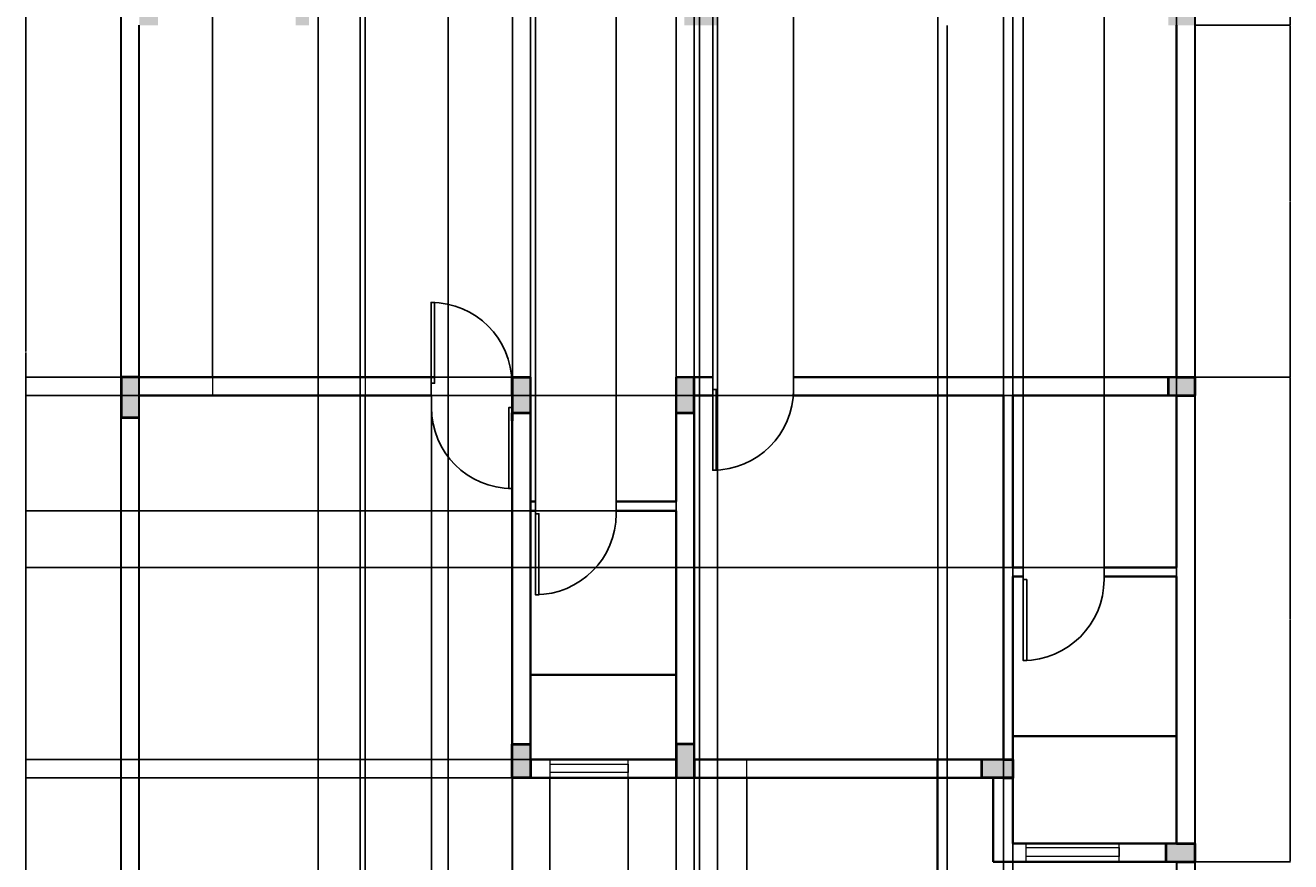
# Model space of a CAD drawing. Units: inches. Extents: x 1210 to 1836, y 84 to 1122.
# Tile 2 of 5: x 1210 to 1836, y 351 to 764. Entities that reach past the tile are written whole.
import ezdxf

# ---------------------------------------------------------------- set-up
doc = ezdxf.new("R2010")
doc.units = ezdxf.units.IN
doc.header["$MEASUREMENT"] = 0
for name, color, linetype, lineweight in [('A-ANNO-DIMS', 2, 'Continuous', 18), ('A-COLS', 7, 'Continuous', 40), ('A-COLS-PATT', 6, 'Continuous', 13), ('A-GLAZ', 4, 'Continuous', 18), ('A-WALL', 7, 'Continuous', 35), ('C-PROP', 32, 'Continuous', 30), ('DOORS', 24, 'Continuous', 25)]:
    doc.layers.add(name, color=color, linetype=linetype, lineweight=lineweight)
doc.styles.get("Standard").update_dxf_attribs({"font": 'arial.ttf'})
doc.dimstyles.get("Standard").update_dxf_attribs({"dimtxt": 0.18, "dimasz": 0.18, "dimexe": 0.18, "dimexo": 0.0625, "dimgap": 0.09, "dimtad": 0, "dimtih": 1, "dimtoh": 1, "dimdec": 4, "dimzin": 0, "dimdsep": 46, "dimtxsty": 'Standard', "dimcen": 0.09, "dimadec": 0, "dimazin": 0, "dimtfac": 1, "dimtdec": 4, "dimtofl": 0, "dimtmove": 0, "dimatfit": 3, "dimfxl": 1, "dimtolj": 1, "dimtzin": 0, "dimarcsym": 0})

# ---------------------------------------------------------------- blocks, each defined once
blk = doc.blocks.new('*U2')
for p, q in [((0, 0), (0, -6)), ((40, 0), (40, -6))]:
    blk.add_line(p, q)
blk.add_lwpolyline([(0, 0), (0, 40), (1.75, 40), (1.75, 0)], close=True)
blk.add_arc((0, 0), 40, 0, 90)
blk = doc.blocks.new('*U5')
for p, q in [((-40, 0), (-40, 6)), ((0, 0), (0, 6))]:
    blk.add_line(p, q)
blk.add_lwpolyline([(0, 0), (0, -40), (-1.75, -40), (-1.75, 0)], close=True)
blk.add_arc((0, 0), 40, 180, 270)
blk = doc.blocks.new('*U4')
for p, q in [((0, 0), (0, 6)), ((40, 0), (40, 6))]:
    blk.add_line(p, q)
blk.add_lwpolyline([(0, 0), (0, -40), (1.75, -40), (1.75, 0)], close=True)
blk.add_arc((0, 0), 40, 270, 0)
blk = doc.blocks.new('*D23')
at = {"layer": 'A-ANNO-DIMS', "color": 0, "lineweight": -2, "transparency": 16777216}
for p, q in [((1257.26, 1074.21), (1209.97, 1074.21)), ((1210.15, 1074.03), (1210.15, 602.9)), ((1210.15, 131.39), (1210.15, 602.53)), ((1257.26, 131.21), (1209.97, 131.21))]:
    blk.add_line(p, q, dxfattribs=at)
at = {"layer": 'A-ANNO-DIMS', "color": 0, "transparency": 16777216}
for points in [[(1210.12, 1074.03), (1210.18, 1074.03), (1210.15, 1074.21)], [(1210.12, 131.39), (1210.18, 131.39), (1210.15, 131.21)]]:
    blk.add_solid(points, dxfattribs=at)
at = {"layer": 'Defpoints', "color": 0, "transparency": 16777216}
for p in [(1210.15, 1074.21), (1257.32, 1074.21), (1257.32, 131.21)]:
    blk.add_point(p, dxfattribs=at)
at = {"layer": 'A-ANNO-DIMS', "color": 0, "transparency": 16777216, "insert": (1210.15, 602.71), "char_height": 0.18, "attachment_point": 5}
blk.add_mtext('\\A1;943', dxfattribs=at)
blk = doc.blocks.new('*D25')
at = {"layer": 'A-ANNO-DIMS', "color": 0, "lineweight": -2, "transparency": 16777216}
for p, q in [((1788.39, 938.21), (1835.68, 938.21)), ((1835.5, 938.03), (1835.5, 851.39)), ((1835.5, 764.39), (1835.5, 851.03)), ((1788.39, 764.21), (1835.68, 764.21))]:
    blk.add_line(p, q, dxfattribs=at)
at = {"layer": 'A-ANNO-DIMS', "color": 0, "transparency": 16777216}
for points in [[(1835.47, 938.03), (1835.53, 938.03), (1835.5, 938.21)], [(1835.47, 764.39), (1835.53, 764.39), (1835.5, 764.21)]]:
    blk.add_solid(points, dxfattribs=at)
at = {"layer": 'Defpoints', "color": 0, "transparency": 16777216}
for p in [(1788.32, 938.21), (1788.32, 764.21), (1835.5, 764.21)]:
    blk.add_point(p, dxfattribs=at)
at = {"layer": 'A-ANNO-DIMS', "color": 0, "transparency": 16777216, "insert": (1835.5, 851.21), "char_height": 0.18, "attachment_point": 5}
blk.add_mtext('\\A1;174', dxfattribs=at)
blk = doc.blocks.new('*D26')
at = {"layer": 'A-ANNO-DIMS', "color": 0, "lineweight": -2, "transparency": 16777216}
for p, q in [((1788.39, 764.21), (1835.68, 764.21)), ((1835.5, 764.03), (1835.5, 677.39)), ((1835.5, 590.39), (1835.5, 677.03)), ((1788.39, 590.21), (1835.68, 590.21))]:
    blk.add_line(p, q, dxfattribs=at)
at = {"layer": 'A-ANNO-DIMS', "color": 0, "transparency": 16777216}
for points in [[(1835.47, 764.03), (1835.53, 764.03), (1835.5, 764.21)], [(1835.47, 590.39), (1835.53, 590.39), (1835.5, 590.21)]]:
    blk.add_solid(points, dxfattribs=at)
at = {"layer": 'Defpoints', "color": 0, "transparency": 16777216}
for p in [(1788.32, 764.21), (1788.32, 590.21), (1835.5, 590.21)]:
    blk.add_point(p, dxfattribs=at)
at = {"layer": 'A-ANNO-DIMS', "color": 0, "transparency": 16777216, "insert": (1835.5, 677.21), "char_height": 0.18, "attachment_point": 5}
blk.add_mtext('\\A1;174', dxfattribs=at)
blk = doc.blocks.new('*D27')
at = {"layer": 'A-ANNO-DIMS', "color": 0, "lineweight": -2, "transparency": 16777216}
for p, q in [((1788.39, 590.21), (1835.68, 590.21)), ((1835.5, 590.03), (1835.5, 470.65)), ((1835.5, 350.89), (1835.5, 470.28)), ((1788.39, 350.71), (1835.68, 350.71))]:
    blk.add_line(p, q, dxfattribs=at)
at = {"layer": 'A-ANNO-DIMS', "color": 0, "transparency": 16777216}
for points in [[(1835.47, 590.03), (1835.53, 590.03), (1835.5, 590.21)], [(1835.47, 350.89), (1835.53, 350.89), (1835.5, 350.71)]]:
    blk.add_solid(points, dxfattribs=at)
at = {"layer": 'Defpoints', "color": 0, "transparency": 16777216}
for p in [(1788.32, 590.21), (1788.32, 350.71), (1835.5, 350.71)]:
    blk.add_point(p, dxfattribs=at)
at = {"layer": 'A-ANNO-DIMS', "color": 0, "transparency": 16777216, "insert": (1835.5, 470.46), "char_height": 0.18, "attachment_point": 5}
blk.add_mtext('\\A1;239.5', dxfattribs=at)
blk = doc.blocks.new('*D36')
at = {"layer": 'A-ANNO-DIMS', "color": 0, "lineweight": -2, "transparency": 16777216}
for p, q in [((1552.32, 840.82), (1552.32, 83.86)), ((1661.32, 840.82), (1661.32, 83.86)), ((1552.5, 84.04), (1606.54, 84.04)), ((1661.14, 84.04), (1607.1, 84.04))]:
    blk.add_line(p, q, dxfattribs=at)
at = {"layer": 'A-ANNO-DIMS', "color": 0, "transparency": 16777216}
for points in [[(1552.5, 84.07), (1552.5, 84.01), (1552.32, 84.04)], [(1661.14, 84.07), (1661.14, 84.01), (1661.32, 84.04)]]:
    blk.add_solid(points, dxfattribs=at)
at = {"layer": 'Defpoints', "color": 0, "transparency": 16777216}
for p in [(1552.32, 840.89), (1661.32, 840.89), (1661.32, 84.04)]:
    blk.add_point(p, dxfattribs=at)
at = {"layer": 'A-ANNO-DIMS', "color": 0, "transparency": 16777216, "insert": (1606.82, 84.04), "char_height": 0.18, "attachment_point": 5}
blk.add_mtext('\\A1;109', dxfattribs=at)
blk = doc.blocks.new('*D39')
at = {"layer": 'A-ANNO-DIMS', "color": 0, "lineweight": -2, "transparency": 16777216}
for p, q in [((1354.82, 773.15), (1354.82, 83.86)), ((1543.32, 773.15), (1543.32, 83.86)), ((1355, 84.04), (1448.69, 84.04)), ((1543.14, 84.04), (1449.46, 84.04))]:
    blk.add_line(p, q, dxfattribs=at)
at = {"layer": 'A-ANNO-DIMS', "color": 0, "transparency": 16777216}
for points in [[(1355, 84.07), (1355, 84.01), (1354.82, 84.04)], [(1543.14, 84.07), (1543.14, 84.01), (1543.32, 84.04)]]:
    blk.add_solid(points, dxfattribs=at)
at = {"layer": 'Defpoints', "color": 0, "transparency": 16777216}
for p in [(1354.82, 773.21), (1543.32, 773.21), (1543.32, 84.04)]:
    blk.add_point(p, dxfattribs=at)
at = {"layer": 'A-ANNO-DIMS', "color": 0, "transparency": 16777216, "insert": (1449.07, 84.04), "char_height": 0.18, "attachment_point": 5}
blk.add_mtext('\\A1;188.5', dxfattribs=at)
blk = doc.blocks.new('*D47')
at = {"layer": 'A-ANNO-DIMS', "color": 0, "lineweight": -2, "transparency": 16777216}
for p, q in [((1375.61, 773.15), (1375.61, 83.86)), ((1419.01, 773.15), (1419.01, 83.86)), ((1375.79, 84.04), (1396.98, 84.04)), ((1418.83, 84.04), (1397.64, 84.04))]:
    blk.add_line(p, q, dxfattribs=at)
at = {"layer": 'A-ANNO-DIMS', "color": 0, "transparency": 16777216}
for points in [[(1375.79, 84.07), (1375.79, 84.01), (1375.61, 84.04)], [(1418.83, 84.07), (1418.83, 84.01), (1419.01, 84.04)]]:
    blk.add_solid(points, dxfattribs=at)
at = {"layer": 'Defpoints', "color": 0, "transparency": 16777216}
for p in [(1375.61, 773.21), (1419.01, 773.21), (1419.01, 84.04)]:
    blk.add_point(p, dxfattribs=at)
at = {"layer": 'A-ANNO-DIMS', "color": 0, "transparency": 16777216, "insert": (1397.31, 84.04), "char_height": 0.18, "attachment_point": 5}
blk.add_mtext('\\A1;43.4', dxfattribs=at)
blk = doc.blocks.new('*D48')
at = {"layer": 'A-ANNO-DIMS', "color": 0, "lineweight": -2, "transparency": 16777216}
for p, q in [((1419.01, 773.15), (1419.01, 83.86)), ((1450.89, 772.94), (1450.89, 83.86)), ((1419.19, 84.04), (1434.55, 84.04)), ((1450.71, 84.04), (1435.34, 84.04))]:
    blk.add_line(p, q, dxfattribs=at)
at = {"layer": 'A-ANNO-DIMS', "color": 0, "transparency": 16777216}
for points in [[(1419.19, 84.07), (1419.19, 84.01), (1419.01, 84.04)], [(1450.71, 84.07), (1450.71, 84.01), (1450.89, 84.04)]]:
    blk.add_solid(points, dxfattribs=at)
at = {"layer": 'Defpoints', "color": 0, "transparency": 16777216}
for p in [(1419.01, 773.21), (1450.89, 773), (1450.89, 84.04)]:
    blk.add_point(p, dxfattribs=at)
at = {"layer": 'A-ANNO-DIMS', "color": 0, "transparency": 16777216, "insert": (1434.95, 84.04), "char_height": 0.18, "attachment_point": 5}
blk.add_mtext('\\A1;31.88', dxfattribs=at)
blk = doc.blocks.new('*D57')
at = {"layer": 'A-ANNO-DIMS', "color": 0, "lineweight": -2, "transparency": 16777216}
for p, q in [((1552.32, 764.15), (1552.32, 83.86)), ((1665.82, 764.15), (1665.82, 83.86)), ((1552.5, 84.04), (1608.69, 84.04)), ((1665.64, 84.04), (1609.46, 84.04))]:
    blk.add_line(p, q, dxfattribs=at)
at = {"layer": 'A-ANNO-DIMS', "color": 0, "transparency": 16777216}
for points in [[(1552.5, 84.07), (1552.5, 84.01), (1552.32, 84.04)], [(1665.64, 84.07), (1665.64, 84.01), (1665.82, 84.04)]]:
    blk.add_solid(points, dxfattribs=at)
at = {"layer": 'Defpoints', "color": 0, "transparency": 16777216}
for p in [(1552.32, 764.21), (1665.82, 764.21), (1665.82, 84.04)]:
    blk.add_point(p, dxfattribs=at)
at = {"layer": 'A-ANNO-DIMS', "color": 0, "transparency": 16777216, "insert": (1609.07, 84.04), "char_height": 0.18, "attachment_point": 5}
blk.add_mtext('\\A1;113.5', dxfattribs=at)
blk = doc.blocks.new('*D59')
at = {"layer": 'A-ANNO-DIMS', "color": 0, "lineweight": -2, "transparency": 16777216}
for p, q in [((1459.82, 443.21), (1459.82, 1121.57)), ((1460, 1121.39), (1495.61, 1121.39)), ((1531.64, 1121.39), (1496.04, 1121.39)), ((1531.82, 443.21), (1531.82, 1121.57))]:
    blk.add_line(p, q, dxfattribs=at)
at = {"layer": 'A-ANNO-DIMS', "color": 0, "transparency": 16777216}
for points in [[(1460, 1121.42), (1460, 1121.36), (1459.82, 1121.39)], [(1531.64, 1121.42), (1531.64, 1121.36), (1531.82, 1121.39)]]:
    blk.add_solid(points, dxfattribs=at)
at = {"layer": 'Defpoints', "color": 0, "transparency": 16777216}
for p in [(1531.82, 1121.39), (1459.82, 443.15), (1531.82, 443.15)]:
    blk.add_point(p, dxfattribs=at)
at = {"layer": 'A-ANNO-DIMS', "color": 0, "transparency": 16777216, "insert": (1495.82, 1121.39), "char_height": 0.18, "attachment_point": 5}
blk.add_mtext('\\A1;72', dxfattribs=at)
blk = doc.blocks.new('*D60')
at = {"layer": 'A-ANNO-DIMS', "color": 0, "lineweight": -2, "transparency": 16777216}
for p, q in [((1540.82, 401.28), (1540.82, 1121.57)), ((1541, 1121.39), (1617.04, 1121.39)), ((1693.64, 1121.39), (1617.6, 1121.39)), ((1693.82, 401.28), (1693.82, 1121.57))]:
    blk.add_line(p, q, dxfattribs=at)
at = {"layer": 'A-ANNO-DIMS', "color": 0, "transparency": 16777216}
for points in [[(1541, 1121.42), (1541, 1121.36), (1540.82, 1121.39)], [(1693.64, 1121.42), (1693.64, 1121.36), (1693.82, 1121.39)]]:
    blk.add_solid(points, dxfattribs=at)
at = {"layer": 'Defpoints', "color": 0, "transparency": 16777216}
for p in [(1693.82, 1121.39), (1540.82, 401.21), (1693.82, 401.21)]:
    blk.add_point(p, dxfattribs=at)
at = {"layer": 'A-ANNO-DIMS', "color": 0, "transparency": 16777216, "insert": (1617.32, 1121.39), "char_height": 0.18, "attachment_point": 5}
blk.add_mtext('\\A1;153', dxfattribs=at)
blk = doc.blocks.new('*D61')
at = {"layer": 'A-ANNO-DIMS', "color": 0, "lineweight": -2, "transparency": 16777216}
for p, q in [((1698.32, 412.85), (1698.32, 1121.57)), ((1698.5, 1121.39), (1738.62, 1121.39)), ((1779.14, 1121.39), (1739.03, 1121.39)), ((1779.32, 412.85), (1779.32, 1121.57))]:
    blk.add_line(p, q, dxfattribs=at)
at = {"layer": 'A-ANNO-DIMS', "color": 0, "transparency": 16777216}
for points in [[(1698.5, 1121.42), (1698.5, 1121.36), (1698.32, 1121.39)], [(1779.14, 1121.42), (1779.14, 1121.36), (1779.32, 1121.39)]]:
    blk.add_solid(points, dxfattribs=at)
at = {"layer": 'Defpoints', "color": 0, "transparency": 16777216}
for p in [(1779.32, 1121.39), (1698.32, 412.79), (1779.32, 412.79)]:
    blk.add_point(p, dxfattribs=at)
at = {"layer": 'A-ANNO-DIMS', "color": 0, "transparency": 16777216, "insert": (1738.82, 1121.39), "char_height": 0.18, "attachment_point": 5}
blk.add_mtext('\\A1;81', dxfattribs=at)
blk = doc.blocks.new('*D62')
at = {"layer": 'A-ANNO-DIMS', "color": 0, "lineweight": -2, "transparency": 16777216}
for p, q in [((1450.76, 590.21), (1209.97, 590.21)), ((1210.15, 590.03), (1210.15, 491.4)), ((1210.15, 392.39), (1210.15, 491.03)), ((1450.76, 392.21), (1209.97, 392.21))]:
    blk.add_line(p, q, dxfattribs=at)
at = {"layer": 'A-ANNO-DIMS', "color": 0, "transparency": 16777216}
for points in [[(1210.12, 590.03), (1210.18, 590.03), (1210.15, 590.21)], [(1210.12, 392.39), (1210.18, 392.39), (1210.15, 392.21)]]:
    blk.add_solid(points, dxfattribs=at)
at = {"layer": 'Defpoints', "color": 0, "transparency": 16777216}
for p in [(1210.15, 590.21), (1450.82, 590.21), (1450.82, 392.21)]:
    blk.add_point(p, dxfattribs=at)
at = {"layer": 'A-ANNO-DIMS', "color": 0, "transparency": 16777216, "insert": (1210.15, 491.21), "char_height": 0.18, "attachment_point": 5}
blk.add_mtext('\\A1;198', dxfattribs=at)
blk = doc.blocks.new('*D63')
at = {"layer": 'A-ANNO-DIMS', "color": 0, "lineweight": -2, "transparency": 16777216}
for p, q in [((1531.76, 524.21), (1209.97, 524.21)), ((1210.15, 524.03), (1210.15, 462.9)), ((1210.15, 401.39), (1210.15, 462.53)), ((1531.76, 401.21), (1209.97, 401.21))]:
    blk.add_line(p, q, dxfattribs=at)
at = {"layer": 'A-ANNO-DIMS', "color": 0, "transparency": 16777216}
for points in [[(1210.12, 524.03), (1210.18, 524.03), (1210.15, 524.21)], [(1210.12, 401.39), (1210.18, 401.39), (1210.15, 401.21)]]:
    blk.add_solid(points, dxfattribs=at)
at = {"layer": 'Defpoints', "color": 0, "transparency": 16777216}
for p in [(1210.15, 524.21), (1531.82, 524.21), (1531.82, 401.21)]:
    blk.add_point(p, dxfattribs=at)
at = {"layer": 'A-ANNO-DIMS', "color": 0, "transparency": 16777216, "insert": (1210.15, 462.71), "char_height": 0.18, "attachment_point": 5}
blk.add_mtext('\\A1;123', dxfattribs=at)
blk = doc.blocks.new('*D64')
at = {"layer": 'A-ANNO-DIMS', "color": 0, "lineweight": -2, "transparency": 16777216}
for p, q in [((1779.26, 581.21), (1209.97, 581.21)), ((1210.15, 581.03), (1210.15, 538.9)), ((1210.15, 496.39), (1210.15, 538.53)), ((1779.26, 496.21), (1209.97, 496.21))]:
    blk.add_line(p, q, dxfattribs=at)
at = {"layer": 'A-ANNO-DIMS', "color": 0, "transparency": 16777216}
for points in [[(1210.12, 581.03), (1210.18, 581.03), (1210.15, 581.21)], [(1210.12, 496.39), (1210.18, 496.39), (1210.15, 496.21)]]:
    blk.add_solid(points, dxfattribs=at)
at = {"layer": 'Defpoints', "color": 0, "transparency": 16777216}
for p in [(1210.15, 581.21), (1779.32, 581.21), (1779.32, 496.21)]:
    blk.add_point(p, dxfattribs=at)
at = {"layer": 'A-ANNO-DIMS', "color": 0, "transparency": 16777216, "insert": (1210.15, 538.71), "char_height": 0.18, "attachment_point": 5}
blk.add_mtext('\\A1;85', dxfattribs=at)
blk = doc.blocks.new('*D65')
at = {"layer": 'A-ANNO-DIMS', "color": 0, "lineweight": -2, "transparency": 16777216}
for p, q in [((1549.93, 581.28), (1549.93, 1121.57)), ((1550.11, 1121.39), (1569.48, 1121.39)), ((1589.64, 1121.39), (1570.27, 1121.39)), ((1589.82, 581.28), (1589.82, 1121.57))]:
    blk.add_line(p, q, dxfattribs=at)
at = {"layer": 'A-ANNO-DIMS', "color": 0, "transparency": 16777216}
for points in [[(1550.11, 1121.42), (1550.11, 1121.36), (1549.93, 1121.39)], [(1589.64, 1121.42), (1589.64, 1121.36), (1589.82, 1121.39)]]:
    blk.add_solid(points, dxfattribs=at)
at = {"layer": 'Defpoints', "color": 0, "transparency": 16777216}
for p in [(1589.82, 1121.39), (1549.93, 581.21), (1589.82, 581.21)]:
    blk.add_point(p, dxfattribs=at)
at = {"layer": 'A-ANNO-DIMS', "color": 0, "transparency": 16777216, "insert": (1569.88, 1121.39), "char_height": 0.18, "attachment_point": 5}
blk.add_mtext('\\A1;39.89', dxfattribs=at)
blk = doc.blocks.new('*D66')
at = {"layer": 'A-ANNO-DIMS', "color": 0, "lineweight": -2, "transparency": 16777216}
for p, q in [((1508.09, 392.15), (1508.09, 83.86)), ((1531.82, 392.15), (1531.82, 83.86)), ((1508.27, 84.04), (1519.56, 84.04)), ((1531.64, 84.04), (1520.35, 84.04))]:
    blk.add_line(p, q, dxfattribs=at)
at = {"layer": 'A-ANNO-DIMS', "color": 0, "transparency": 16777216}
for points in [[(1508.27, 84.07), (1508.27, 84.01), (1508.09, 84.04)], [(1531.64, 84.07), (1531.64, 84.01), (1531.82, 84.04)]]:
    blk.add_solid(points, dxfattribs=at)
at = {"layer": 'Defpoints', "color": 0, "transparency": 16777216}
for p in [(1508.09, 392.21), (1531.82, 392.21), (1531.82, 84.04)]:
    blk.add_point(p, dxfattribs=at)
at = {"layer": 'A-ANNO-DIMS', "color": 0, "transparency": 16777216, "insert": (1519.96, 84.04), "char_height": 0.18, "attachment_point": 5}
blk.add_mtext('\\A1;23.73', dxfattribs=at)
blk = doc.blocks.new('*D67')
at = {"layer": 'A-ANNO-DIMS', "color": 0, "lineweight": -2, "transparency": 16777216}
for p, q in [((1469.4, 392.15), (1469.4, 83.86)), ((1508.09, 392.15), (1508.09, 83.86)), ((1469.58, 84.04), (1488.42, 84.04)), ((1507.91, 84.04), (1489.07, 84.04))]:
    blk.add_line(p, q, dxfattribs=at)
at = {"layer": 'A-ANNO-DIMS', "color": 0, "transparency": 16777216}
for points in [[(1469.58, 84.07), (1469.58, 84.01), (1469.4, 84.04)], [(1507.91, 84.07), (1507.91, 84.01), (1508.09, 84.04)]]:
    blk.add_solid(points, dxfattribs=at)
at = {"layer": 'Defpoints', "color": 0, "transparency": 16777216}
for p in [(1469.4, 392.21), (1508.09, 392.21), (1508.09, 84.04)]:
    blk.add_point(p, dxfattribs=at)
at = {"layer": 'A-ANNO-DIMS', "color": 0, "transparency": 16777216, "insert": (1488.75, 84.04), "char_height": 0.18, "attachment_point": 5}
blk.add_mtext('\\A1;38.7', dxfattribs=at)
blk = doc.blocks.new('*D68')
at = {"layer": 'A-ANNO-DIMS', "color": 0, "lineweight": -2, "transparency": 16777216}
for p, q in [((1540.82, 392.15), (1540.82, 83.86)), ((1566.82, 392.15), (1566.82, 83.86)), ((1541, 84.04), (1553.42, 84.04)), ((1566.64, 84.04), (1554.22, 84.04))]:
    blk.add_line(p, q, dxfattribs=at)
at = {"layer": 'A-ANNO-DIMS', "color": 0, "transparency": 16777216}
for points in [[(1541, 84.07), (1541, 84.01), (1540.82, 84.04)], [(1566.64, 84.07), (1566.64, 84.01), (1566.82, 84.04)]]:
    blk.add_solid(points, dxfattribs=at)
at = {"layer": 'Defpoints', "color": 0, "transparency": 16777216}
for p in [(1540.82, 392.21), (1566.82, 392.21), (1566.82, 84.04)]:
    blk.add_point(p, dxfattribs=at)
at = {"layer": 'A-ANNO-DIMS', "color": 0, "transparency": 16777216, "insert": (1553.82, 84.04), "char_height": 0.18, "attachment_point": 5}
blk.add_mtext('\\A1;25.99', dxfattribs=at)
blk = doc.blocks.new('*D69')
at = {"layer": 'A-ANNO-DIMS', "color": 0, "lineweight": -2, "transparency": 16777216}
for p, q in [((1566.82, 392.15), (1566.82, 83.86)), ((1660.99, 392.15), (1660.99, 83.86)), ((1567, 84.04), (1613.51, 84.04)), ((1660.81, 84.04), (1614.29, 84.04))]:
    blk.add_line(p, q, dxfattribs=at)
at = {"layer": 'A-ANNO-DIMS', "color": 0, "transparency": 16777216}
for points in [[(1567, 84.07), (1567, 84.01), (1566.82, 84.04)], [(1660.81, 84.07), (1660.81, 84.01), (1660.99, 84.04)]]:
    blk.add_solid(points, dxfattribs=at)
at = {"layer": 'Defpoints', "color": 0, "transparency": 16777216}
for p in [(1566.82, 392.21), (1660.99, 392.21), (1660.99, 84.04)]:
    blk.add_point(p, dxfattribs=at)
at = {"layer": 'A-ANNO-DIMS', "color": 0, "transparency": 16777216, "insert": (1613.9, 84.04), "char_height": 0.18, "attachment_point": 5}
blk.add_mtext('\\A1;94.17', dxfattribs=at)
blk = doc.blocks.new('*D72')
at = {"layer": 'A-ANNO-DIMS', "color": 0, "lineweight": -2, "transparency": 16777216}
for p, q in [((1257.32, 590.28), (1257.32, 1121.57)), ((1257.5, 1121.39), (1279.44, 1121.39)), ((1302.31, 1121.39), (1280.37, 1121.39)), ((1302.49, 590.28), (1302.49, 1121.57))]:
    blk.add_line(p, q, dxfattribs=at)
at = {"layer": 'A-ANNO-DIMS', "color": 0, "transparency": 16777216}
for points in [[(1257.5, 1121.42), (1257.5, 1121.36), (1257.32, 1121.39)], [(1302.31, 1121.42), (1302.31, 1121.36), (1302.49, 1121.39)]]:
    blk.add_solid(points, dxfattribs=at)
at = {"layer": 'Defpoints', "color": 0, "transparency": 16777216}
for p in [(1302.49, 1121.39), (1257.32, 590.21), (1302.49, 590.21)]:
    blk.add_point(p, dxfattribs=at)
at = {"layer": 'A-ANNO-DIMS', "color": 0, "transparency": 16777216, "insert": (1279.91, 1121.39), "char_height": 0.18, "attachment_point": 5}
blk.add_mtext('\\A1;45.165', dxfattribs=at)
blk = doc.blocks.new('*D73')
at = {"layer": 'A-ANNO-DIMS', "color": 0, "lineweight": -2, "transparency": 16777216}
for p, q in [((1302.49, 590.28), (1302.49, 1121.57)), ((1302.67, 1121.39), (1339.91, 1121.39)), ((1377.81, 1121.39), (1340.56, 1121.39)), ((1377.99, 590.28), (1377.99, 1121.57))]:
    blk.add_line(p, q, dxfattribs=at)
at = {"layer": 'A-ANNO-DIMS', "color": 0, "transparency": 16777216}
for points in [[(1302.67, 1121.42), (1302.67, 1121.36), (1302.49, 1121.39)], [(1377.81, 1121.42), (1377.81, 1121.36), (1377.99, 1121.39)]]:
    blk.add_solid(points, dxfattribs=at)
at = {"layer": 'Defpoints', "color": 0, "transparency": 16777216}
for p in [(1377.99, 1121.39), (1302.49, 590.21), (1377.99, 590.21)]:
    blk.add_point(p, dxfattribs=at)
at = {"layer": 'A-ANNO-DIMS', "color": 0, "transparency": 16777216, "insert": (1340.24, 1121.39), "char_height": 0.18, "attachment_point": 5}
blk.add_mtext('\\A1;75.5', dxfattribs=at)
blk = doc.blocks.new('*D74')
at = {"layer": 'A-ANNO-DIMS', "color": 0, "lineweight": -2, "transparency": 16777216}
for p, q in [((1377.99, 581.15), (1377.99, 83.86)), ((1410.82, 581.15), (1410.82, 83.86)), ((1378.17, 84.04), (1394.01, 84.04)), ((1410.64, 84.04), (1394.8, 84.04))]:
    blk.add_line(p, q, dxfattribs=at)
at = {"layer": 'A-ANNO-DIMS', "color": 0, "transparency": 16777216}
for points in [[(1378.17, 84.07), (1378.17, 84.01), (1377.99, 84.04)], [(1410.64, 84.07), (1410.64, 84.01), (1410.82, 84.04)]]:
    blk.add_solid(points, dxfattribs=at)
at = {"layer": 'Defpoints', "color": 0, "transparency": 16777216}
for p in [(1377.99, 581.21), (1410.82, 581.21), (1410.82, 84.04)]:
    blk.add_point(p, dxfattribs=at)
at = {"layer": 'A-ANNO-DIMS', "color": 0, "transparency": 16777216, "insert": (1394.4, 84.04), "char_height": 0.18, "attachment_point": 5}
blk.add_mtext('\\A1;32.84', dxfattribs=at)
blk = doc.blocks.new('*D75')
at = {"layer": 'A-ANNO-DIMS', "color": 0, "lineweight": -2, "transparency": 16777216}
for p, q in [((1410.82, 575.15), (1410.82, 83.86)), ((1450.82, 575.15), (1450.82, 83.86)), ((1411, 84.04), (1430.6, 84.04)), ((1450.64, 84.04), (1431.05, 84.04))]:
    blk.add_line(p, q, dxfattribs=at)
at = {"layer": 'A-ANNO-DIMS', "color": 0, "transparency": 16777216}
for points in [[(1411, 84.07), (1411, 84.01), (1410.82, 84.04)], [(1450.64, 84.07), (1450.64, 84.01), (1450.82, 84.04)]]:
    blk.add_solid(points, dxfattribs=at)
at = {"layer": 'Defpoints', "color": 0, "transparency": 16777216}
for p in [(1410.82, 575.21), (1450.82, 575.21), (1450.82, 84.04)]:
    blk.add_point(p, dxfattribs=at)
at = {"layer": 'A-ANNO-DIMS', "color": 0, "transparency": 16777216, "insert": (1430.82, 84.04), "char_height": 0.18, "attachment_point": 5}
blk.add_mtext('\\A1;40', dxfattribs=at)
blk = doc.blocks.new('*D76')
at = {"layer": 'A-ANNO-DIMS', "color": 0, "lineweight": -2, "transparency": 16777216}
for p, q in [((1462.25, 528.78), (1462.25, 1121.57)), ((1462.43, 1121.39), (1482.03, 1121.39)), ((1502.07, 1121.39), (1482.47, 1121.39)), ((1502.25, 528.78), (1502.25, 1121.57))]:
    blk.add_line(p, q, dxfattribs=at)
at = {"layer": 'A-ANNO-DIMS', "color": 0, "transparency": 16777216}
for points in [[(1462.43, 1121.42), (1462.43, 1121.36), (1462.25, 1121.39)], [(1502.07, 1121.42), (1502.07, 1121.36), (1502.25, 1121.39)]]:
    blk.add_solid(points, dxfattribs=at)
at = {"layer": 'Defpoints', "color": 0, "transparency": 16777216}
for p in [(1502.25, 1121.39), (1462.25, 528.71), (1502.25, 528.71)]:
    blk.add_point(p, dxfattribs=at)
at = {"layer": 'A-ANNO-DIMS', "color": 0, "transparency": 16777216, "insert": (1482.25, 1121.39), "char_height": 0.18, "attachment_point": 5}
blk.add_mtext('\\A1;40', dxfattribs=at)
blk = doc.blocks.new('*D77')
at = {"layer": 'A-ANNO-DIMS', "color": 0, "lineweight": -2, "transparency": 16777216}
for p, q in [((1703.49, 496.28), (1703.49, 1121.57)), ((1703.67, 1121.39), (1723.26, 1121.39)), ((1743.31, 1121.39), (1723.71, 1121.39)), ((1743.49, 496.28), (1743.49, 1121.57))]:
    blk.add_line(p, q, dxfattribs=at)
at = {"layer": 'A-ANNO-DIMS', "color": 0, "transparency": 16777216}
for points in [[(1703.67, 1121.42), (1703.67, 1121.36), (1703.49, 1121.39)], [(1743.31, 1121.42), (1743.31, 1121.36), (1743.49, 1121.39)]]:
    blk.add_solid(points, dxfattribs=at)
at = {"layer": 'Defpoints', "color": 0, "transparency": 16777216}
for p in [(1743.49, 1121.39), (1703.49, 496.21), (1743.49, 496.21)]:
    blk.add_point(p, dxfattribs=at)
at = {"layer": 'A-ANNO-DIMS', "color": 0, "transparency": 16777216, "insert": (1723.49, 1121.39), "char_height": 0.18, "attachment_point": 5}
blk.add_mtext('\\A1;40', dxfattribs=at)
blk = doc.blocks.new('*D78')
at = {"layer": 'A-ANNO-DIMS', "color": 0, "lineweight": -2, "transparency": 16777216}
for p, q in [((1693.82, 581.15), (1693.82, 83.86)), ((1698.32, 581.15), (1698.32, 83.86)), ((1694, 84.04), (1695.82, 84.04)), ((1698.14, 84.04), (1696.33, 84.04))]:
    blk.add_line(p, q, dxfattribs=at)
at = {"layer": 'A-ANNO-DIMS', "color": 0, "transparency": 16777216}
for points in [[(1694, 84.07), (1694, 84.01), (1693.82, 84.04)], [(1698.14, 84.07), (1698.14, 84.01), (1698.32, 84.04)]]:
    blk.add_solid(points, dxfattribs=at)
at = {"layer": 'Defpoints', "color": 0, "transparency": 16777216}
for p in [(1693.82, 581.21), (1698.32, 581.21), (1698.32, 84.04)]:
    blk.add_point(p, dxfattribs=at)
at = {"layer": 'A-ANNO-DIMS', "color": 0, "transparency": 16777216, "insert": (1696.07, 84.04), "char_height": 0.18, "attachment_point": 5}
blk.add_mtext('\\A1;4.5', dxfattribs=at)

msp = doc.modelspace()

# ---------------------------------------------------------------- hatches: boundary and pattern name
at = {"layer": 'A-COLS-PATT'}
h = msp.add_hatch(color=256, dxfattribs=at)
h.dxf.hatch_style = 1
h.paths.add_polyline_path([(1266.3239, 938.214), (1257.3239, 938.214), (1257.3239, 929.4573), (1257.3239, 923.2025), (1266.3239, 923.2025)])
h.paths.add_polyline_path([(1350.3239, 929.214), (1350.3239, 938.214), (1339.1886, 938.214), (1339.1886, 929.214)])
h.paths.add_polyline_path([(1559.1961, 929.214), (1559.1961, 938.214), (1542.8626, 938.214), (1542.8626, 929.214), (1543.3239, 929.214)])
h.paths.add_polyline_path([(1771.5139, 938.214), (1771.5139, 929.214), (1788.3239, 929.214), (1788.3239, 938.214)])
h.paths.add_polyline_path([(1788.3239, 764.214), (1788.3239, 773.214), (1775.2119, 773.214), (1775.2119, 764.214)])
h.paths.add_polyline_path([(1552.3239, 764.214), (1552.3239, 773.214), (1543.3239, 773.214), (1535.8494, 773.197), (1535.8494, 764.214)])
h.paths.add_polyline_path([(1275.5217, 782.2138), (1272.7843, 782.2138), (1266.3239, 782.2138), (1266.3239, 764.214), (1275.5217, 764.214)])
h.paths.add_polyline_path([(1350.2372, 764.214), (1350.3239, 773.214), (1343.6352, 773.214), (1343.6352, 764.214)])
h.paths.add_polyline_path([(1257.3239, 570.3846), (1266.3239, 570.3846), (1266.3239, 590.214), (1257.3239, 590.214)])
h.paths.add_polyline_path([(1450.8239, 572.5809), (1459.8239, 572.5809), (1459.8239, 590.214), (1458.3239, 590.214), (1450.8239, 590.214)])
h.paths.add_polyline_path([(1531.8239, 572.5809), (1540.8239, 572.5809), (1540.8239, 590.214), (1531.8239, 590.214)])
h.paths.add_polyline_path([(1450.8239, 392.214), (1459.8239, 392.214), (1459.8239, 401.214), (1459.8239, 408.7866), (1450.8239, 408.7866)])
h.paths.add_polyline_path([(1531.8239, 392.214), (1540.8239, 392.214), (1540.8239, 401.214), (1540.8239, 408.7866), (1531.8239, 408.7866)])
h.paths.add_polyline_path([(1682.9725, 401.214), (1682.9725, 392.214), (1698.3239, 392.214), (1698.3239, 401.214), (1693.8239, 401.214)])
h.paths.add_polyline_path([(1774.197, 350.714), (1779.3239, 350.714), (1788.3239, 350.714), (1788.3239, 359.714), (1779.3239, 359.714), (1774.197, 359.714)])
h.paths.add_polyline_path([(1779.3239, 590.214), (1775.4485, 590.214), (1775.4485, 581.214), (1779.3239, 581.214), (1788.3239, 581.214), (1788.3239, 590.214)])

# ---------------------------------------------------------------- linework, layer by layer
at = {"layer": 'A-COLS'}
for p, q in [((1266.3239, 590.214), (1257.3239, 590.214)), ((1257.3239, 590.214), (1257.3239, 570.3846)), ((1450.4926, 590.214), (1458.3239, 590.214)), ((1450.8239, 581.214), (1450.8239, 590.214)), ((1450.8239, 590.214), (1450.8239, 568.7267)), ((1458.3239, 590.214), (1459.8239, 590.214)), ((1540.8239, 572.5809), (1540.8239, 590.214)), ((1775.4485, 581.214), (1775.4485, 590.214)), ((1779.3239, 590.214), (1788.3239, 590.214)), ((1788.3239, 590.214), (1788.3239, 581.1742)), ((1450.6052, 581.214), (1450.8239, 581.214)), ((1779.3239, 581.214), (1788.3239, 581.214)), ((1257.3239, 570.3846), (1266.3239, 570.3846)), ((1450.8239, 568.7267), (1450.8239, 572.5809)), ((1450.8239, 572.5809), (1459.8239, 572.5809)), ((1531.8239, 572.5809), (1540.8239, 572.5809)), ((1450.8239, 392.214), (1450.8239, 408.7866)), ((1450.8239, 408.7866), (1459.8239, 408.7866)), ((1540.8239, 408.7866), (1531.8239, 408.7866)), ((1531.8239, 408.7866), (1531.8239, 392.214)), ((1459.8239, 401.214), (1459.8239, 392.214)), ((1540.8239, 401.214), (1540.8239, 392.214)), ((1682.9725, 392.214), (1682.9725, 401.214)), ((1693.8239, 401.214), (1698.3239, 401.214)), ((1698.3239, 401.214), (1698.3239, 392.0825)), ((1459.8239, 392.214), (1450.8239, 392.214)), ((1698.3239, 392.214), (1682.9725, 392.214)), ((1693.8239, 392.214), (1698.3239, 392.214)), ((1774.197, 350.714), (1774.197, 359.714)), ((1779.3239, 359.714), (1788.3239, 359.714)), ((1788.3239, 359.714), (1788.3239, 350.8323)), ((1779.3239, 350.714), (1788.3239, 350.714))]:
    msp.add_line(p, q, dxfattribs=at)
at = {"layer": 'A-GLAZ'}
for p, q in [((1302.4894, 590.214), (1302.4894, 581.214)), ((1378.2066, 581.5192), (1378.2066, 590.5192)), ((1302.4894, 581.214), (1377.9853, 581.214)), ((1469.397, 401.214), (1469.397, 392.214)), ((1508.0938, 392.214), (1508.0938, 401.214)), ((1566.8155, 392.214), (1566.8155, 401.214)), ((1660.9867, 392.214), (1660.9867, 401.214)), ((1469.397, 398.974), (1508.0938, 398.974)), ((1508.0938, 394.8322), (1469.397, 394.8322)), ((1508.0938, 398.974), (1508.0938, 394.8322)), ((1704.8288, 359.714), (1704.8288, 350.714)), ((1704.8288, 359.714), (1704.8288, 357.757)), ((1704.8288, 357.757), (1750.8976, 357.757)), ((1750.8976, 350.714), (1750.8976, 359.714)), ((1750.8976, 357.757), (1750.8976, 355.214)), ((1750.8976, 353.3014), (1704.8288, 353.3014)), ((1704.8288, 350.714), (1750.8976, 350.714)), ((1750.8976, 355.214), (1750.8976, 353.3014))]:
    msp.add_line(p, q, dxfattribs=at)
at = {"layer": 'A-WALL'}
for p, q in [((1779.3239, 764.214), (1779.3239, 590.214)), ((1266.3239, 590.214), (1412.3552, 590.214)), ((1377.9853, 590.214), (1394.3053, 590.214)), ((1459.8239, 401.214), (1459.8239, 590.214)), ((1531.8239, 590.214), (1549.9335, 590.214)), ((1531.8239, 590.214), (1531.8239, 528.714)), ((1589.9335, 590.214), (1779.3239, 590.214)), ((1266.3239, 581.214), (1410.8239, 581.214)), ((1450.8239, 581.214), (1450.8239, 392.214)), ((1540.8239, 581.214), (1540.8239, 401.214)), ((1540.8239, 581.214), (1549.9335, 581.214)), ((1589.8208, 581.214), (1693.8239, 581.214)), ((1693.8239, 581.214), (1693.8239, 401.214)), ((1698.3239, 581.214), (1698.3239, 496.214)), ((1698.3239, 581.214), (1779.3239, 581.214)), ((1779.3239, 581.214), (1779.3239, 496.214)), ((1459.8239, 528.714), (1462.2498, 528.714)), ((1502.2498, 528.714), (1531.8239, 528.714)), ((1459.8239, 524.214), (1462.2498, 524.214)), ((1502.2498, 524.214), (1531.8239, 524.214)), ((1531.8239, 524.214), (1531.8239, 401.214)), ((1698.3239, 496.214), (1703.4865, 496.214)), ((1743.4865, 496.214), (1779.3239, 496.214)), ((1698.3239, 491.714), (1703.4865, 491.714)), ((1698.3239, 359.714), (1698.3239, 491.714)), ((1743.4865, 491.714), (1779.3239, 491.714)), ((1779.3239, 359.714), (1779.3239, 491.714)), ((1459.8239, 443.1518), (1531.8239, 443.1518)), ((1698.3239, 412.7914), (1779.3239, 412.7914)), ((1459.8239, 401.214), (1531.8239, 401.214)), ((1540.8239, 401.214), (1693.8239, 401.214)), ((1531.8239, 392.214), (1450.8239, 392.214)), ((1531.8239, 392.214), (1693.8239, 392.214)), ((1688.7218, 350.714), (1688.7218, 392.214)), ((1698.3239, 359.714), (1779.3239, 359.714)), ((1693.8239, 350.714), (1688.7218, 350.714)), ((1693.8239, 350.714), (1779.3239, 350.714))]:
    msp.add_line(p, q, dxfattribs=at)
at = {"layer": 'C-PROP'}
for p, q in [((1257.3239, 131.214), (1257.3239, 1074.214)), ((1788.3239, 1074.214), (1788.3239, 131.214)), ((1266.3239, 140.214), (1266.3239, 764.214)), ((1779.3239, 350.714), (1779.3239, 140.214))]:
    msp.add_line(p, q, dxfattribs=at)

# ---------------------------------------------------------------- block references
at = {"layer": 'DOORS'}
for name, p in [('*U2', (1410.6052, 587.214)), ('*U4', (1549.9335, 584.214)), ('*U5', (1450.8239, 575.214)), ('*U4', (1462.2498, 522.714)), ('*U4', (1703.4865, 490.214))]:
    msp.add_blockref(name, p, dxfattribs=at)

# ---------------------------------------------------------------- dimensions: what is measured, and where the dimension line sits
at = {"layer": 'A-ANNO-DIMS'}
for base, p1, p2, override, picture, middle in [((1302.4894, 1121.38901), (1257.32392, 590.21401), (1302.4894, 590.21401), {"dimdec": 3, "dimlfac": 1, "dimrnd": 0, "dimzin": 0, "dimdsep": 46, "dimlunit": 2}, '*D72', (1279.90666, 1121.38901)), ((1377.9853, 1121.389), (1302.4894, 590.214), (1377.9853, 590.214), {"dimdec": 1, "dimlfac": 1, "dimrnd": 0, "dimzin": 0, "dimdsep": 46, "dimlunit": 2}, '*D73', (1340.2374, 1121.389)), ((1531.8239, 1121.389), (1459.8239, 443.1518), (1531.8239, 443.1518), {"dimdec": 0, "dimlfac": 1, "dimrnd": 0, "dimzin": 0, "dimdsep": 46, "dimlunit": 2}, '*D59', (1495.8239, 1121.389)), ((1502.2498, 1121.389), (1462.2498, 528.714), (1502.2498, 528.714), {"dimdec": 0, "dimlfac": 1, "dimrnd": 0, "dimzin": 0, "dimdsep": 46, "dimlunit": 2}, '*D76', (1482.2498, 1121.389)), ((1693.8239, 1121.389), (1540.8239, 401.214), (1693.8239, 401.214), {"dimdec": 0, "dimlfac": 1, "dimrnd": 0, "dimzin": 0, "dimdsep": 46, "dimlunit": 2}, '*D60', (1617.3239, 1121.389)), ((1589.8208, 1121.389), (1549.9335, 581.214), (1589.8208, 581.214), {"dimdec": 2, "dimlfac": 1, "dimrnd": 0, "dimzin": 0, "dimdsep": 46, "dimlunit": 2}, '*D65', (1569.8772, 1121.389)), ((1779.3239, 1121.389), (1698.3239, 412.7914), (1779.3239, 412.7914), {"dimdec": 0, "dimlfac": 1, "dimrnd": 0, "dimzin": 0, "dimdsep": 46, "dimlunit": 2}, '*D61', (1738.8239, 1121.389)), ((1743.4865, 1121.389), (1703.4865, 496.214), (1743.4865, 496.214), {"dimdec": 0, "dimlfac": 1, "dimrnd": 0, "dimzin": 0, "dimdsep": 46, "dimlunit": 2}, '*D77', (1723.4865, 1121.389)), ((1661.3239, 84.039), (1552.3239, 840.8861), (1661.3239, 840.8861), {"dimdec": 0, "dimlfac": 1, "dimrnd": 0, "dimzin": 0, "dimdsep": 46, "dimlunit": 2}, '*D36', (1606.8239, 84.039)), ((1543.3239, 84.039), (1354.8239, 773.214), (1543.3239, 773.214), {"dimdec": 1, "dimlfac": 1, "dimrnd": 0, "dimzin": 0, "dimdsep": 46, "dimlunit": 2}, '*D39', (1449.0739, 84.039)), ((1419.0081, 84.039), (1375.6096, 773.214), (1419.0081, 773.214), {"dimdec": 1, "dimlfac": 1, "dimrnd": 0, "dimzin": 0, "dimdsep": 46, "dimlunit": 2}, '*D47', (1397.3088, 84.039)), ((1450.8864, 84.039), (1419.0081, 773.214), (1450.8864, 773.0031), {"dimdec": 2, "dimlfac": 1, "dimrnd": 0, "dimzin": 0, "dimdsep": 46, "dimlunit": 2}, '*D48', (1434.9472, 84.039)), ((1665.8239, 84.039), (1552.3239, 764.214), (1665.8239, 764.214), {"dimdec": 1, "dimlfac": 1, "dimrnd": 0, "dimzin": 0, "dimdsep": 46, "dimlunit": 2}, '*D57', (1609.0739, 84.039)), ((1410.8239, 84.039), (1377.9853, 581.214), (1410.8239, 581.214), {"dimdec": 2, "dimlfac": 1, "dimrnd": 0, "dimzin": 0, "dimdsep": 46, "dimlunit": 2}, '*D74', (1394.4046, 84.039)), ((1698.3239, 84.039), (1693.8239, 581.214), (1698.3239, 581.214), {"dimdec": 1, "dimlfac": 1, "dimrnd": 0, "dimzin": 0, "dimdsep": 46, "dimlunit": 2}, '*D78', (1696.0739, 84.039)), ((1450.8239, 84.039), (1410.8239, 575.214), (1450.8239, 575.214), {"dimdec": 0, "dimlfac": 1, "dimrnd": 0, "dimzin": 0, "dimdsep": 46, "dimlunit": 2}, '*D75', (1430.8239, 84.039)), ((1508.0938, 84.039), (1469.397, 392.214), (1508.0938, 392.214), {"dimdec": 1, "dimlfac": 1, "dimrnd": 0, "dimzin": 0, "dimdsep": 46, "dimlunit": 2}, '*D67', (1488.7454, 84.039)), ((1531.8239, 84.039), (1508.0938, 392.214), (1531.8239, 392.214), {"dimdec": 2, "dimlfac": 1, "dimrnd": 0, "dimzin": 0, "dimdsep": 46, "dimlunit": 2}, '*D66', (1519.9588, 84.039)), ((1566.8155, 84.039), (1540.8239, 392.214), (1566.8155, 392.214), {"dimdec": 2, "dimlfac": 1, "dimrnd": 0, "dimzin": 0, "dimdsep": 46, "dimlunit": 2}, '*D68', (1553.8197, 84.039)), ((1660.9867, 84.039), (1566.8155, 392.214), (1660.9867, 392.214), {"dimdec": 2, "dimlfac": 1, "dimrnd": 0, "dimzin": 0, "dimdsep": 46, "dimlunit": 2}, '*D69', (1613.9011, 84.039))]:
    dim = msp.add_linear_dim(base=base, p1=p1, p2=p2, dimstyle='Standard', override=override, dxfattribs=at)
    dim.commit()
    dim.dimension.update_dxf_attribs({"geometry": picture, "text_midpoint": middle})
for base, p1, p2, override, picture, middle in [((1210.1489, 1074.214), (1257.3239, 131.214), (1257.3239, 1074.214), {"dimdec": 0, "dimlfac": 1, "dimrnd": 0, "dimzin": 0, "dimdsep": 46, "dimlunit": 2}, '*D23', (1210.1489, 602.714)), ((1835.4989, 764.214), (1788.3239, 938.214), (1788.3239, 764.214), {"dimdec": 0, "dimlfac": 1, "dimrnd": 0, "dimzin": 0, "dimdsep": 46, "dimlunit": 2}, '*D25', (1835.4989, 851.214)), ((1835.4989, 590.214), (1788.3239, 764.214), (1788.3239, 590.214), {"dimdec": 0, "dimlfac": 1, "dimrnd": 0, "dimzin": 0, "dimdsep": 46, "dimlunit": 2}, '*D26', (1835.4989, 677.214)), ((1210.1489, 590.214), (1450.8239, 392.214), (1450.8239, 590.214), {"dimdec": 0, "dimlfac": 1, "dimrnd": 0, "dimzin": 0, "dimdsep": 46, "dimlunit": 2}, '*D62', (1210.1489, 491.214)), ((1835.4989, 350.714), (1788.3239, 590.214), (1788.3239, 350.714), {"dimdec": 1, "dimlfac": 1, "dimrnd": 0, "dimzin": 0, "dimdsep": 46, "dimlunit": 2}, '*D27', (1835.4989, 470.464)), ((1210.1489, 581.214), (1779.3239, 496.214), (1779.3239, 581.214), {"dimdec": 0, "dimlfac": 1, "dimrnd": 0, "dimzin": 0, "dimdsep": 46, "dimlunit": 2}, '*D64', (1210.1489, 538.714)), ((1210.1489, 524.214), (1531.8239, 401.214), (1531.8239, 524.214), {"dimdec": 0, "dimlfac": 1, "dimrnd": 0, "dimzin": 0, "dimdsep": 46, "dimlunit": 2}, '*D63', (1210.1489, 462.714))]:
    dim = msp.add_linear_dim(base=base, p1=p1, p2=p2, angle=90, dimstyle='Standard', override=override, dxfattribs=at)
    dim.commit()
    dim.dimension.update_dxf_attribs({"geometry": picture, "text_midpoint": middle})

doc.saveas('drawing.dxf')
